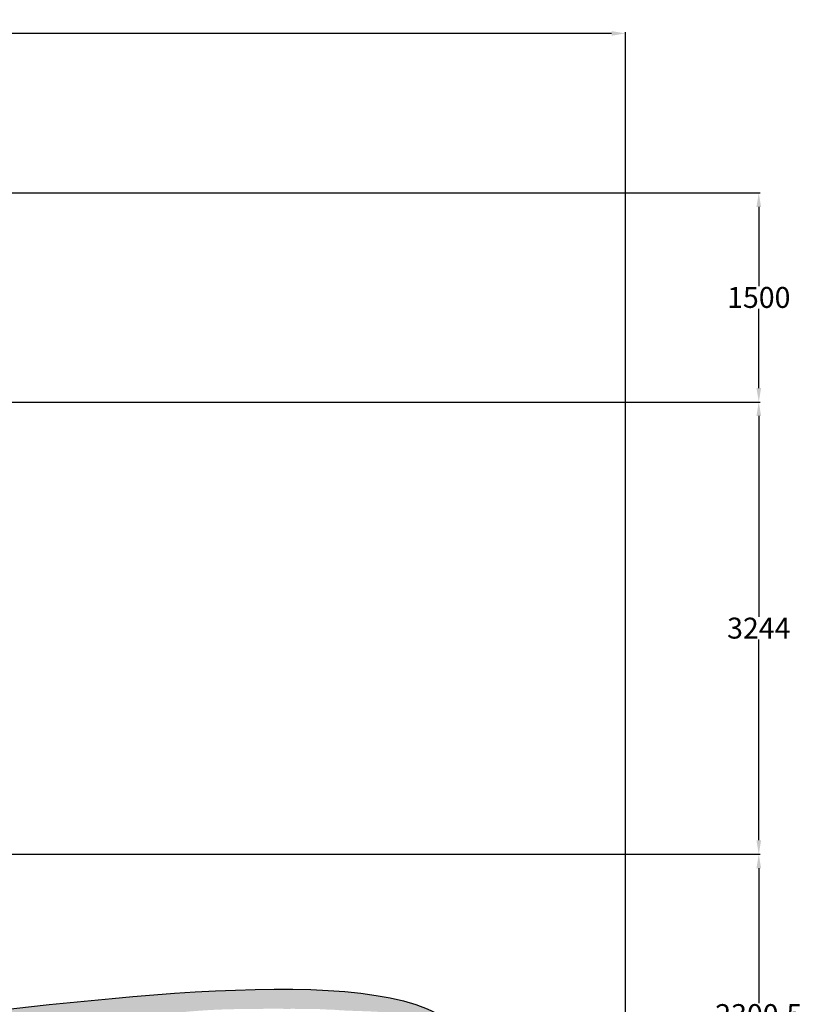
# Model space of a CAD drawing. Units: millimetres. Extents: x 11032 to 26788, y 3406 to 24505.
# Tile 78 of 78: x 21051 to 26666, y 17443 to 24505. Entities that reach past the tile are written whole.
import ezdxf

# ---------------------------------------------------------------- set-up
doc = ezdxf.new("R2010")
doc.units = ezdxf.units.MM
doc.header["$MEASUREMENT"] = 0
doc.layers.add('A-ANNO-DIMS', color=2, linetype='Continuous', lineweight=18)
doc.layers.add('A-ROOF', color=7, linetype='Continuous', lineweight=30)
doc.layers.add('A-ROOF-PATT', color=9, linetype='Continuous', lineweight=13, true_color=0xc7c8ca)
doc.styles.get("Standard").update_dxf_attribs({"font": 'arial.ttf'})
doc.dimstyles.get("Standard").update_dxf_attribs({"dimtxt": 150, "dimasz": 100, "dimexe": 10, "dimexo": 5, "dimgap": 5, "dimtad": 0, "dimtih": 1, "dimtoh": 1, "dimdec": 0, "dimzin": 0, "dimdsep": 46, "dimtxsty": 'Standard', "dimcen": 0.09, "dimadec": 0, "dimazin": 0, "dimtfac": 1, "dimtdec": 0, "dimtofl": 0, "dimtmove": 0, "dimatfit": 3, "dimfxl": 1, "dimtolj": 1, "dimtzin": 0, "dimarcsym": 0})

# ---------------------------------------------------------------- blocks, each defined once
blk = doc.blocks.new('*D36')
at = {"layer": 'A-ANNO-DIMS', "color": 0, "lineweight": -2, "transparency": 16777216}
for p, q in [((12301.3, 17115.9), (12301.3, 24416.9)), ((12401.3, 24406.9), (18569.2, 24406.9)), ((25297.4, 24406.9), (19129.5, 24406.9)), ((25397.4, 4466.4), (25397.4, 24416.9))]:
    blk.add_line(p, q, dxfattribs=at)
at = {"layer": 'A-ANNO-DIMS', "color": 0, "transparency": 16777216}
for points in [[(12401.3, 24423.5), (12401.3, 24390.2), (12301.3, 24406.9)], [(25297.4, 24423.5), (25297.4, 24390.2), (25397.4, 24406.9)]]:
    blk.add_solid(points, dxfattribs=at)
at = {"layer": 'Defpoints', "color": 0, "transparency": 16777216}
for p in [(25397.4, 24406.9), (12301.3, 17110.9), (25397.4, 4461.4)]:
    blk.add_point(p, dxfattribs=at)
at = {"layer": 'A-ANNO-DIMS', "color": 0, "transparency": 16777216, "insert": (18849.3, 24406.9), "char_height": 150, "attachment_point": 5}
blk.add_mtext('\\A1;13096', dxfattribs=at)
blk = doc.blocks.new('*D45')
at = {"layer": 'A-ANNO-DIMS', "color": 0, "lineweight": -2, "transparency": 16777216}
for p, q in [((13792.4, 18518.9), (26363.9, 18518.9)), ((26353.9, 18418.9), (26353.9, 17450.3)), ((26353.9, 16318.4), (26353.9, 17287)), ((22902.4, 16218.4), (26363.9, 16218.4))]:
    blk.add_line(p, q, dxfattribs=at)
at = {"layer": 'A-ANNO-DIMS', "color": 0, "transparency": 16777216}
for points in [[(26337.2, 18418.9), (26370.6, 18418.9), (26353.9, 18518.9)], [(26337.2, 16318.4), (26370.6, 16318.4), (26353.9, 16218.4)]]:
    blk.add_solid(points, dxfattribs=at)
at = {"layer": 'Defpoints', "color": 0, "transparency": 16777216}
for p in [(13787.4, 18518.9), (26353.9, 18518.9), (22897.4, 16218.4)]:
    blk.add_point(p, dxfattribs=at)
at = {"layer": 'A-ANNO-DIMS', "color": 0, "transparency": 16777216, "insert": (26353.9, 17368.7), "char_height": 150, "attachment_point": 5}
blk.add_mtext('\\A1;2300.5', dxfattribs=at)
blk = doc.blocks.new('*D46')
at = {"layer": 'A-ANNO-DIMS', "color": 0, "lineweight": -2, "transparency": 16777216}
for p, q in [((18497.2, 21762.9), (26363.9, 21762.9)), ((26353.9, 21662.9), (26353.9, 20222.6)), ((26353.9, 18618.9), (26353.9, 20059.3)), ((13792.4, 18518.9), (26363.9, 18518.9))]:
    blk.add_line(p, q, dxfattribs=at)
at = {"layer": 'A-ANNO-DIMS', "color": 0, "transparency": 16777216}
for points in [[(26337.2, 21662.9), (26370.6, 21662.9), (26353.9, 21762.9)], [(26337.2, 18618.9), (26370.6, 18618.9), (26353.9, 18518.9)]]:
    blk.add_solid(points, dxfattribs=at)
at = {"layer": 'Defpoints', "color": 0, "transparency": 16777216}
for p in [(18492.2, 21762.9), (26353.9, 21762.9), (13787.4, 18518.9)]:
    blk.add_point(p, dxfattribs=at)
at = {"layer": 'A-ANNO-DIMS', "color": 0, "transparency": 16777216, "insert": (26353.9, 20140.9), "char_height": 150, "attachment_point": 5}
blk.add_mtext('\\A1;3244', dxfattribs=at)
blk = doc.blocks.new('*D47')
at = {"layer": 'A-ANNO-DIMS', "color": 0, "lineweight": -2, "transparency": 16777216}
for p, q in [((18559.6, 23262.9), (26363.9, 23262.9)), ((26353.9, 23162.9), (26353.9, 22594.5)), ((26353.9, 21862.9), (26353.9, 22431.4)), ((18497.2, 21762.9), (26363.9, 21762.9))]:
    blk.add_line(p, q, dxfattribs=at)
at = {"layer": 'A-ANNO-DIMS', "color": 0, "transparency": 16777216}
for points in [[(26337.2, 23162.9), (26370.6, 23162.9), (26353.9, 23262.9)], [(26337.2, 21862.9), (26370.6, 21862.9), (26353.9, 21762.9)]]:
    blk.add_solid(points, dxfattribs=at)
at = {"layer": 'Defpoints', "color": 0, "transparency": 16777216}
for p in [(18554.6, 23262.9), (26353.9, 23262.9), (18492.2, 21762.9)]:
    blk.add_point(p, dxfattribs=at)
at = {"layer": 'A-ANNO-DIMS', "color": 0, "transparency": 16777216, "insert": (26353.9, 22512.9), "char_height": 150, "attachment_point": 5}
blk.add_mtext('\\A1;1500', dxfattribs=at)

msp = doc.modelspace()

# ---------------------------------------------------------------- hatches: boundary and pattern name
at = {"layer": 'A-ROOF-PATT'}
h = msp.add_hatch(color=256, dxfattribs=at)
edge = h.paths.add_edge_path()
edge.add_spline(control_points=[(18514.126, 17063.566), (18809.773, 17038.521), (19288.07, 16988.339), (19761.843, 17020.464), (19965.955, 17031.58)], knot_values=[0, 0, 0, 0, 871.48115533, 1383.18424693, 1383.18424693, 1383.18424693, 1383.18424693], degree=3, periodic=0)
edge.add_spline(control_points=[(19965.955, 17031.58), (20122.484, 17046.068), (20408.011, 17091.181), (20910.567, 17150.246), (21440.234, 17310.172), (21915.866, 17351.508), (22364.272, 17406.622), (22705.353, 17409.356), (22912.577, 17410.967), (22981.194, 17409.426)], knot_values=[0, 0, 0, 0, 414.81784697, 1085.22788952, 1556.54039253, 2003.31216232, 2520.51919616, 2899.47011217, 3092.27759325, 3092.27759325, 3092.27759325, 3092.27759325], degree=3, periodic=0)
edge.add_spline(control_points=[(22981.194, 17409.426), (23026.355, 17412.719), (23070.675, 17406.134), (23179.968, 17412.17), (23244.326, 17403.734), (23304.873, 17403.391)], knot_values=[11756.28081343, 11756.28081343, 11756.28081343, 11756.28081343, 11879.15309498, 11879.15309498, 12065.87545546, 12065.87545546, 12065.87545546, 12065.87545546], degree=3, periodic=0)
edge.add_spline(control_points=[(23304.873, 17403.391), (23443.416, 17391.278), (23687.5, 17400.339), (23988.629, 17323.661), (24193.084, 17226.949), (24257.37, 17136.735), (24279.347, 17098.191)], knot_values=[0, 0, 0, 0, 412.75172359, 727.19040018, 931.86025321, 1064.01641738, 1064.01641738, 1064.01641738, 1064.01641738], degree=3, periodic=0)
edge.add_spline(control_points=[(24279.347, 17098.191), (24276.632, 17112.026), (24103.56, 17784.539), (21679.83, 17482.933), (20092.886, 17311.864), (19886.51, 17298.161)], knot_values=[9435.32329041, 9435.32329041, 9435.32329041, 9435.32329041, 9511.54858978, 13244.41643911, 13837.11981978, 13837.11981978, 13837.11981978, 13837.11981978], degree=3, periodic=0)
edge.add_spline(control_points=[(19886.51, 17298.161), (19770.33, 17290.447), (19654.15, 17282.732), (19537.97, 17275.018), (19460.41, 17269.868), (19382.851, 17264.718), (19305.291, 17259.568)], knot_values=[8878.9087223, 8878.9087223, 8878.9087223, 8878.9087223, 9212.57342317, 9212.57342317, 9212.57342317, 9435.32303857, 9435.32303857, 9435.32303857, 9435.32303857], degree=3, periodic=0)
edge.add_spline(control_points=[(19305.291, 17259.568), (19183.371, 17255.041), (18919.19, 17257.277), (18655.158, 17260.282), (18513.182, 17263.662)], knot_values=[568.98430855, 568.98430855, 568.98430855, 568.98430855, 934.97323186, 1361.07600794, 1361.07600794, 1361.07600794, 1361.07600794], degree=3, periodic=0)
edge.add_line((18513.182, 17263.662), (18514.126, 17063.566))

# ---------------------------------------------------------------- linework, layer by layer
at = {"layer": 'A-ROOF'}
msp.add_open_spline([(19305.291, 17259.568), (19382.851, 17264.718), (19460.41, 17269.868), (19537.97, 17275.018), (19654.15, 17282.732), (19770.33, 17290.447), (19886.51, 17298.161), (19886.51, 17298.161), (19886.51, 17298.161), (19886.51, 17298.161), (20092.886, 17311.864), (21679.83, 17482.933), (25498.5, 17958.124), (23655.645, 15804.534), (22897.404, 14361.22)], degree=3, knots=[8878.9087223, 8878.9087223, 8878.9087223, 8878.9087223, 9101.65833771, 9101.65833771, 9101.65833771, 9435.32303857, 9435.32303857, 9435.32303857, 9435.32329041, 9435.32329041, 9435.32329041, 10028.02667108, 13760.8945204, 16370.50452639, 16370.50452639, 16370.50452639, 16370.50452639], dxfattribs=at)

# ---------------------------------------------------------------- dimensions: what is measured, and where the dimension line sits
at = {"layer": 'A-ANNO-DIMS'}
dim = msp.add_linear_dim(base=(25397.404, 24406.858), p1=(12301.265, 17110.885), p2=(25397.404, 4461.399), dimstyle='Standard', override={"dimdec": 0, "dimlfac": 1, "dimrnd": 0, "dimzin": 0, "dimdsep": 46, "dimlunit": 2}, dxfattribs=at)
dim.commit()
dim.dimension.update_dxf_attribs({"geometry": '*D36', "text_midpoint": (18849.334, 24406.858)})
for base, p1, p2, override, picture, middle in [((26353.904, 23262.945), (18492.19, 21762.945), (18554.563, 23262.945), {"dimdec": 0, "dimlfac": 1, "dimrnd": 0, "dimzin": 0, "dimdsep": 46, "dimlunit": 2}, '*D47', (26353.904, 22512.945)), ((26353.904, 21762.945), (13787.367, 18518.925), (18492.19, 21762.945), {"dimdec": 0, "dimlfac": 1, "dimrnd": 0, "dimzin": 0, "dimdsep": 46, "dimlunit": 2}, '*D46', (26353.904, 20140.935)), ((26353.904, 18518.925), (22897.404, 16218.44), (13787.367, 18518.925), {"dimdec": 1, "dimlfac": 1, "dimrnd": 0, "dimzin": 0, "dimdsep": 46, "dimlunit": 2}, '*D45', (26353.904, 17368.682))]:
    dim = msp.add_linear_dim(base=base, p1=p1, p2=p2, angle=90, dimstyle='Standard', override=override, dxfattribs=at)
    dim.commit()
    dim.dimension.update_dxf_attribs({"geometry": picture, "text_midpoint": middle})

doc.saveas('drawing.dxf')
